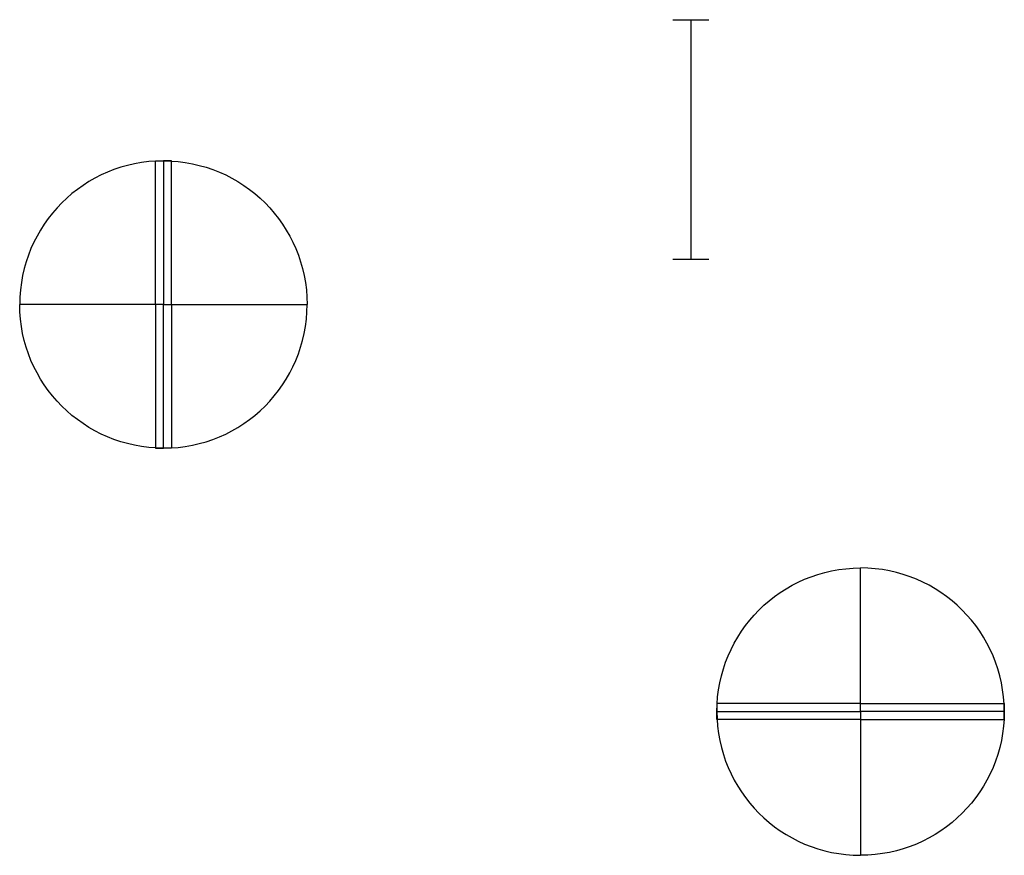
# Model space of a CAD drawing. Units: inches. Extents: x -349 to 9053, y 635 to 6001.
# Tile 1 of 7: x -349 to -103, y 906 to 1116. Entities that reach past the tile are written whole.
import ezdxf

# ---------------------------------------------------------------- set-up
doc = ezdxf.new("R2010")
doc.units = ezdxf.units.IN
doc.layers.add('A-DOOR', color=3, linetype='Continuous', lineweight=25)
doc.layers.add('A-GLAZ', color=4, linetype='Continuous', lineweight=25)

# ---------------------------------------------------------------- blocks, each defined once
blk = doc.blocks.new('DOOR-36IN-SWING-WITH-THRESHOLD')
blk.add_line((0, 0), (0, -36))
blk.add_lwpolyline([(-36, 0), (0, 0), (0, -2), (-36, -2)], close=True)
blk.add_arc((0, 0), 36, 180, 270)
blk = doc.blocks.new('WIN-60IN')
for p, q in [((0, -4.5), (0, 4.5)), ((60, -4.5), (60, 4.5)), ((0, 0), (60, 0))]:
    blk.add_line(p, q)

msp = doc.modelspace()

# ---------------------------------------------------------------- block references
at = {"layer": 'A-DOOR'}
for p, rotation in [((-313.4824, 1044.3112), 270.0000000000004), ((-313.4824, 1044.3112), 89.99999999999996), ((-138.8369, 942.3038), 180)]:
    msp.add_blockref('DOOR-36IN-SWING-WITH-THRESHOLD', p, dxfattribs=dict(at, rotation=rotation))
at = {"layer": 'A-DOOR', "extrusion": (0, 0, -1), "zscale": -1}
for p, rotation in [((313.4824, 1044.3112), 270.0000000000003), ((313.4824, 1044.3112), 90.00000000000003), ((138.8369, 942.3038), 180)]:
    msp.add_blockref('DOOR-36IN-SWING-WITH-THRESHOLD', p, dxfattribs=dict(at, rotation=rotation))
at = {"layer": 'A-DOOR'}
msp.add_blockref('DOOR-36IN-SWING-WITH-THRESHOLD', (-138.8369, 942.3038), dxfattribs=at)
at = {"layer": 'A-DOOR', "extrusion": (0, 0, -1), "zscale": -1}
msp.add_blockref('DOOR-36IN-SWING-WITH-THRESHOLD', (138.8369, 942.3038), dxfattribs=at)
at = {"layer": 'A-GLAZ', "rotation": 269.9999999999998}
msp.add_blockref('WIN-60IN', (-181.3366, 1115.6735), dxfattribs=at)

doc.saveas('drawing.dxf')
